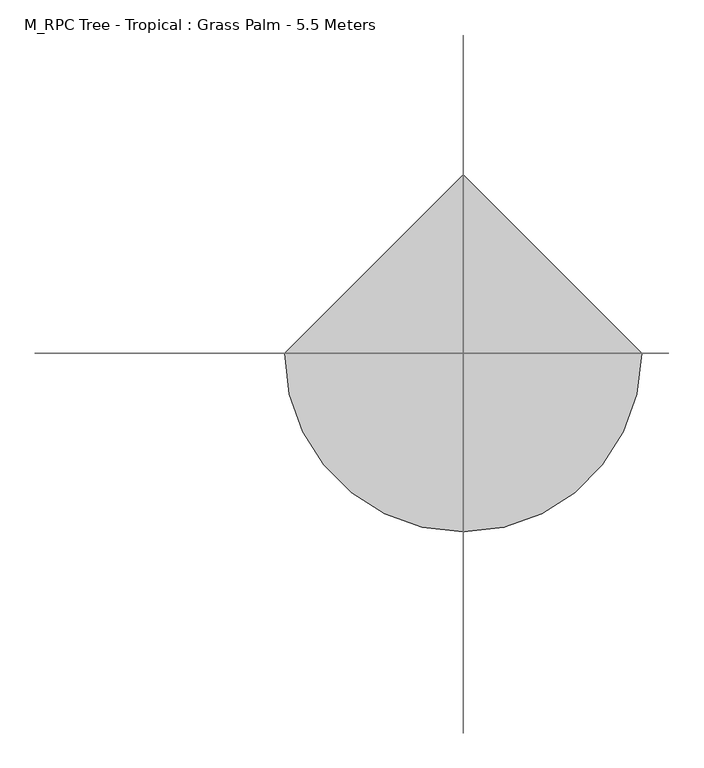
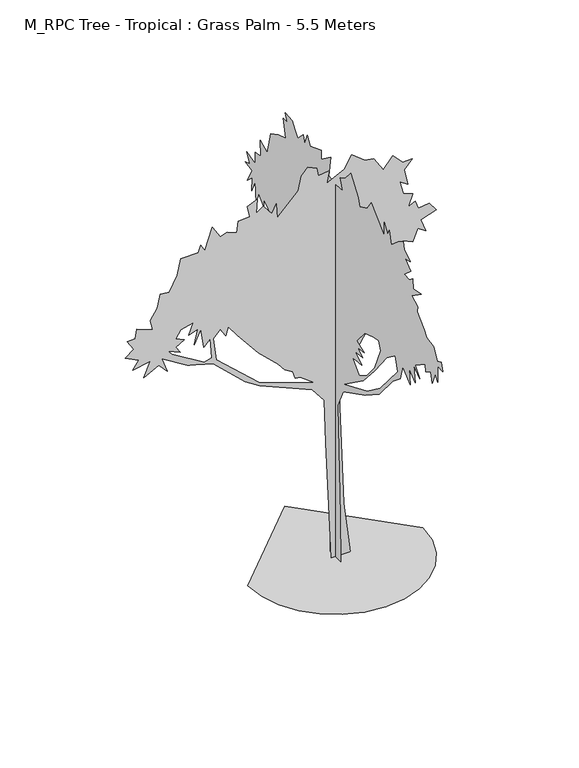
"""IFC4 building model written with IfcOpenShell, lengths in millimetres: geographic element geometry, M_RPC Tree - Tropical : Grass Palm - 5.5 Meters."""

from ifc_helpers import new_model, si_unit, origin, place, context, project, spatial, triangles, source, transform, mapped, element, save


def m_rpc_tree_tropical_grass_palm_5_5_meters_0f61173e(model_context):
    return source(origin(), model_context, "Body", "Tessellation", [
        triangles([(198.5121563, -0.0004669, 0.000137), (109.5820013, -0.0002641, 696.282209), (43.8536913, 0.0002053, 2386.4069527), (410.3796021, 0.0003086, 2969.8983719), (572.0261307, 0.000406, 3417.6646454), (609.3777389, 0.0004587, 3632.4192696), (721.4325634, 0.000452, 3669.7733849), (656.0666405, 0.0004949, 3791.1807999), (749.4469145, 0.0005265, 3959.2618195), (777.4587221, 0.0005019, 3884.5535889), (880.1763622, 0.0005321, 4052.6346085), (1010.9057373, 0.0004946, 3987.2711563), (1076.2717329, 0.0005304, 4155.3521759), (1178.9867569, 0.0004946, 4080.6439453), (1113.6233774, 0.0005527, 4258.0697433), (1319.0559689, 0.0005395, 4323.4331955), (1225.6756222, 0.0005866, 4444.8150307), (1085.6090263, 0.0006027, 4426.1507629), (1042.0062372, 0.0006404, 4540.8870735), (954.8795786, 0.0006402, 4491.5142151), (1010.9057373, 0.0006749, 4650.2504562), (889.3481134, 0.0007069, 4700.3869308), (842.8247177, 0.0007612, 4874.3754387), (945.5397417, 0.0007279, 4808.9864067), (898.8508764, 0.0007933, 5023.7666107), (1001.5685165, 0.0008083, 5135.8289566), (880.1763622, 0.0008266, 5135.8289566), (749.4469145, 0.0008819, 5266.5558609), (628.0548328, 0.0008596, 5117.1393997), (505.3182475, 0.0009317, 5314.2482986), (385.2705606, 0.0009547, 5331.919313), (217.1877242, 0.0010181, 5471.9909958), (114.4714012, 0.000988, 5303.9099762), (-109.6373213, 0.0009913, 5191.8476303), (-81.6239785, 0.0010303, 5350.5838715), (-221.6916826, 0.0010463, 5331.919313), (-240.3675048, 0.0010796, 5443.9816589), (-361.7593503, 0.0011132, 5500.0003326), (-445.7998964, 0.0011005, 5406.6275436), (-483.1515046, 0.0010553, 5219.8569672), (-753.9502007, 0.0010201, 4939.7386002), (-772.6247149, 0.0010762, 5135.8289566), (-828.653417, 0.0010542, 5023.7666107), (-940.7082779, 0.0011092, 5163.8382935), (-1034.0860811, 0.0011055, 5098.4748413), (-1015.4090235, 0.0011535, 5285.2204193), (-1146.140942, 0.001158, 5229.2017456), (-1118.1265909, 0.0011131, 5079.7852844), (-1267.5330963, 0.0011332, 5070.4655045), (-1286.2076832, 0.0010954, 4921.0490433), (-1407.5996922, 0.0011264, 4967.747937), (-1500.9775681, 0.0011329, 4939.7386002), (-1603.6951355, 0.0011941, 5107.8196198), (-1706.4127029, 0.0011309, 4818.3314758), (-1753.1017136, 0.0011633, 4911.7042648), (-1790.4532127, 0.0011436, 4818.3314758), (-2014.5604637, 0.0011774, 4818.3314758), (-2061.249329, 0.0011261, 4603.5768517), (-2163.9668964, 0.0010882, 4407.4609154), (-2285.3590508, 0.0011091, 4416.8059845), (-2322.7106953, 0.0010665, 4239.3798958), (-2416.0885712, 0.0010425, 4099.3337929), (-2382.6964233, 0.0010016, 3967.2572617), (-2593.5117531, 0.0010541, 4043.2895393), (-2612.1760208, 0.0010239, 3921.9077042), (-2714.8935883, 0.0010369, 3912.5629257), (-2630.8658684, 0.0009886, 3781.8360214), (-2742.9029251, 0.0009827, 3697.7827217), (-2565.5024162, 0.0009305, 3604.4099327), (-2640.1853577, 0.0009113, 3492.3475868), (-2416.0885712, 0.0008902, 3539.0464806), (-2500.1287903, 0.0008496, 3342.9564148), (-2304.0361084, 0.0008479, 3445.6739822), (-2191.9813202, 0.000798, 3324.2665672), (-2266.6819931, 0.0008626, 3520.3822128), (-1932.5900311, 0.0007558, 3313.3428154), (-1590.273571, 0.0006787, 3219.8174194), (-1172.1055635, 0.0005081, 2824.7595566), (-982.5363207, 0.0004459, 2701.1877388), (-300.5056764, 0.0002631, 2407.6914093), (-143.5331084, 0.0001855, 2209.3782234), (-126.2243993, 2.09e-05, 1613.6007809), (-53.6101361, -0.0004288, 0.000137), (-1500.9775681, 0.0008979, 3660.4538956), (-1426.2768951, 0.0008562, 3548.3915497), (-1398.2624714, 0.0008824, 3660.4538956), (-1276.8703171, 0.0008209, 3501.6923653), (-1004.3554831, 0.0003611, 3164.2318588), (-746.3927404, 0.0005806, 2912.4030441), (-661.4253977, 0.0005394, 2808.0812141), (-557.8547573, 0.0005067, 2745.340567), (-520.5031128, 0.0004731, 2642.6229996), (-455.1371535, 0.0004607, 2633.2779305), (-268.3816016, 0.0003944, 2493.2088638), (-997.3532215, 0.0005761, 2756.6459816), (-1553.2123158, 0.0007974, 3261.8314247), (-1594.3579147, 0.0008866, 3567.0558174), (-2023.9003006, 0.0008876, 3529.7017021), (-2079.9263866, 0.0009189, 3613.7550018), (-1967.8715984, 0.0009197, 3679.118454), (-2079.9263866, 0.0009519, 3735.136837), (-2014.5604637, 0.00097, 3837.8544044), (-1855.8166649, 0.0009561, 3875.2085197), (-1911.8453671, 0.000924, 3725.8173477), (-1795.9710445, 0.0009167, 3763.5025475), (-1842.3900135, 0.0008704, 3567.2848732), (-1753.1017136, 0.0009076, 3753.8266846), (-1715.750069, 0.0008309, 3492.3475868), (-1631.7095592, 0.0008411, 3576.4008865), (-1612.4492523, 0.0007652, 3307.9445984), (-1712.8319332, 0.0007726, 3279.4007011), (-2135.952618, 0.000907, 3539.0464806), (-2182.6440994, 0.0009293, 3595.0651543), (0.1967722, -126.2945259, 0.0001596), (0.196734, -114.2887362, 634.3486347), (0.1967033, -52.2143547, 2120.548035), (0.1966846, -175.5378682, 2379.5675446), (0.1966095, -673.1974989, 2636.9445671), (0.1965211, -992.9715849, 2843.0418709), (0.1965145, -1302.1785107, 3208.1809204), (0.196489, -1470.9471336, 3342.9564148), (0.1964806, -1526.9732197, 3548.3915497), (0.1964552, -1695.0542393, 3398.9747978), (0.1964594, -1667.0424316, 3604.4099327), (0.1964383, -1807.1091728, 3492.372876), (0.1964439, -1769.7575283, 3716.4725693), (0.1964228, -1909.8242695, 3613.7550018), (0.1964383, -1807.1091728, 3735.136837), (0.1964044, -2031.2188946, 3884.5535889), (0.1964016, -2049.8934814, 3791.1807999), (0.1963861, -2152.6110489, 3847.1994736), (0.1963805, -2189.9600773, 3716.4725693), (0.1963706, -2255.3261456, 3884.5535889), (0.1963607, -2320.6920685, 3809.8450676), (0.1963607, -2320.6920685, 4033.9447609), (0.1963438, -2432.7443859, 4024.6252716), (0.1963495, -2395.3953575, 4136.6623283), (0.1963636, -2302.0150108, 4089.9887238), (0.1963748, -2227.3117218, 4248.7249649), (0.1963988, -2068.5705391, 4276.7340111), (0.1964073, -2012.5418369, 4351.4425323), (0.1963912, -1853.7980381, 4500.8592842), (0.1963898, -1863.1354042, 4575.541935), (0.1964095, -1732.4058838, 4650.2504562), (0.1963771, -1947.175914, 4799.6669174), (0.1964053, -1760.4203075, 4762.3128021), (0.1964067, -1751.0829414, 4893.0397064), (0.196418, -1676.3797977, 4837.0213234), (0.1964349, -1564.3248642, 4846.340522), (0.1964137, -1704.3916054, 4967.747937), (0.1964321, -1583.0019218, 5070.4655045), (0.1964151, -1695.0542393, 5098.4748413), (0.1964363, -1554.9876434, 5182.5028519), (0.1964391, -1536.3105858, 5275.9006393), (0.196456, -1424.2556522, 5210.5371872), (0.19648, -1265.5118534, 5070.4655045), (0.196487, -1218.8229881, 5238.546524), (0.1964927, -1181.4714163, 5163.8382935), (0.1964639, -1106.7706707, 5285.2204193), (0.196504, -1106.7706707, 5098.4748413), (0.1964895, -937.1364029, 5255.9634842), (0.196509, -807.9577326, 5369.2734283), (0.196521, -728.2942812, 5249.9283875), (0.1965471, -555.8361669, 5163.8382935), (0.1965527, -518.4845223, 5266.5558609), (0.1965781, -350.4035028, 5500.0003326), (0.1965964, -229.0103492, 5359.9286499), (0.1966148, -107.618204, 5294.5651978), (0.1966063, -163.6456435, 5145.173735), (0.1966288, -14.2397308, 5135.8289566), (0.1966528, 144.5038522, 5163.8382935), (0.1966472, 107.1527437, 5443.9816589), (0.1966782, 312.5858983, 5294.5651978), (0.1966782, 312.5858983, 5415.9473236), (0.1967163, 564.707464, 5322.5745346), (0.1967261, 630.0734596, 5434.6368805), (0.196736, 695.4368391, 5275.9006393), (0.1967402, 723.4511902, 5378.6182068), (0.1967586, 844.8433445, 5257.2110825), (0.1967684, 910.2093401, 5322.5745346), (0.1967783, 975.5727922, 5425.2921021), (0.1967622, 1134.3165184, 5434.6368805), (0.1967952, 1087.6276531, 5331.919313), (0.1968083, 1174.4359446, 5339.303746), (0.1967995, 1115.6420042, 5098.4748413), (0.1968263, 1293.0603172, 5033.1113892), (0.1968508, 1455.9824947, 4950.7135117), (0.1968629, 1535.8446259, 4640.9053871), (0.1968869, 1694.5882793, 4715.6139084), (0.1968855, 1685.2510586, 4500.8592842), (0.1969038, 1806.6432129, 4482.1694366), (0.1969038, 1806.6432129, 4323.4331955), (0.1969334, 2002.7386562, 4370.1068001), (0.1969223, 1928.9571133, 4250.787339), (0.1969389, 2038.9214767, 4214.579084), (0.1969151, 1881.3465019, 4183.3615128), (0.196932, 1993.4012901, 3987.2711563), (0.1969137, 1872.0091358, 4089.9887238), (0.1969165, 1890.6837227, 3903.2178566), (0.1969038, 1806.6432129, 4080.6439453), (0.196901, 1787.968626, 3800.5002892), (0.1968925, 1731.9399239, 3959.2618195), (0.1968756, 1619.8851357, 3847.1994736), (0.1968756, 1619.8851357, 3949.917041), (0.196869, 1310.8614109, 3745.6530556), (0.1968099, 919.5466335, 3632.4192696), (0.1967908, 792.5526409, 3237.1576401), (0.1967898, 785.995919, 3141.3913925), (0.1967733, 676.7623249, 3072.1575371), (0.1967987, 844.8433445, 2941.4309235), (0.1967817, 732.7884836, 2978.7850388), (0.1968246, 751.4629978, 2782.6946823), (0.1968091, 648.7479738, 2913.4215866), (0.1968063, 630.0734596, 2679.9771149), (0.1968021, 602.0590722, 2782.6946823), (0.1967978, 574.0447211, 2679.9771149), (0.1967908, 527.3558195, 2848.0581345), (0.1967866, 499.3414684, 2689.2966042), (0.1967837, 480.6669542, 2614.6136627), (0.1967781, 443.3153097, 2745.340567), (0.1967682, 377.9493505, 2661.2872673), (0.1967491, 251.276432, 2499.1212936), (0.1966956, 162.3905602, 2114.1747322), (0.1967682, 112.1317639, 1064.5480299), (0.1968089, 116.4897555, 0.0001162), (0.1965757, -631.608831, 2807.9538963), (0.196537, -888.1940414, 3104.5465485), (0.1964954, -1163.6294821, 3449.6205437), (0.1964659, -1358.8922001, 3595.0651543), (0.1964574, -1414.9184315, 3408.3195763), (0.1965169, -1021.2762526, 2939.164492), (0.1965619, -722.832478, 2719.5465019), (0.1966421, -191.6594859, 2493.2088638), (0.1966027, -453.1185631, 2988.104528), (0.1965815, -593.187775, 2997.4493065), (0.1966027, -453.1185631, 3100.1668739), (0.1965773, -621.2021261, 3118.8567215), (0.1965942, -509.0072302, 3191.7316338), (0.1965716, -658.5512272, 3212.2295105), (0.196597, -490.4701713, 3277.5929626), (0.1965705, -666.1620998, 3486.8985008), (0.1965392, -873.3236555, 3557.7363281), (0.1965223, -985.3785164, 3576.4008865), (0.1965161, -1026.231328, 3465.2294746), (0.1965365, -891.2878206, 3143.9121689), (0.1965617, -724.2889297, 2942.0163528), (0.19659, -537.1590729, 2820.0235085), (0.1966111, -397.0924044, 2978.7850388), (-1142.7569189, 0.0, 0.000137), (-1112.5425568, -261.8891381, 0.0001838), (-1026.4879257, -502.3944798, 0.0002268), (-891.4833029, -714.6206245, 0.0002648), (-714.4239796, -891.6799479, 0.0002965), (-502.195255, -1026.6845707, 0.0), (-261.692475, -1112.7392017, 1.54e-05), (0.1967389, -1142.9535639, 2.08e-05), (262.0858013, -1112.7392017, 1.54e-05), (502.5911611, -1026.6845707, 0.0), (714.8172695, -891.6799479, 0.0002965), (891.8765928, -714.6206245, 0.0002648), (1026.8812157, -502.3919363, 0.0002268), (1112.9358467, -261.8891381, 0.0001838), (1143.1502089, 9.99e-05, 0.000137), (0.1965231, 1142.9535639, 0.0002532)], [[95, 110, 96], [86, 3, 87], [87, 3, 88], [88, 3, 89], [106, 105, 107], [89, 3, 90], [90, 3, 91], [74, 73, 75], [42, 41, 43], [14, 13, 15], [98, 113, 99], [72, 71, 73], [96, 110, 97], [110, 109, 97], [70, 69, 71], [24, 23, 25], [26, 25, 27], [85, 84, 86], [55, 54, 56], [53, 52, 54], [104, 103, 105], [10, 9, 11], [108, 107, 109], [100, 99, 101], [46, 45, 47], [47, 45, 48], [66, 65, 67], [68, 67, 69], [16, 15, 17], [17, 15, 18], [35, 34, 36], [73, 71, 75], [64, 63, 65], [7, 6, 8], [3, 86, 4], [19, 18, 20], [32, 31, 33], [1, 83, 2], [83, 82, 2], [2, 82, 3], [82, 81, 3], [28, 27, 29], [12, 11, 13], [81, 80, 3], [4, 86, 5], [5, 86, 6], [21, 20, 22], [44, 43, 45], [27, 25, 29], [25, 23, 29], [60, 59, 61], [99, 113, 101], [49, 48, 50], [57, 56, 58], [6, 86, 8], [38, 37, 39], [37, 36, 39], [39, 36, 40], [36, 34, 40], [65, 63, 67], [67, 63, 69], [69, 63, 71], [71, 63, 75], [92, 91, 93], [91, 3, 93], [93, 3, 94], [3, 80, 94], [80, 79, 94], [94, 79, 95], [79, 78, 95], [95, 78, 110], [78, 77, 110], [110, 77, 111], [77, 76, 111], [111, 76, 112], [76, 75, 112], [112, 75, 113], [75, 63, 113], [113, 63, 101], [101, 63, 102], [97, 109, 84], [109, 107, 84], [8, 86, 9], [63, 62, 102], [62, 61, 102], [61, 59, 102], [102, 59, 103], [59, 58, 103], [58, 56, 103], [56, 54, 103], [18, 15, 20], [15, 13, 20], [13, 11, 20], [54, 52, 103], [52, 51, 103], [51, 50, 103], [103, 50, 105], [105, 50, 107], [107, 50, 84], [84, 50, 86], [86, 50, 9], [50, 48, 9], [48, 45, 9], [40, 34, 41], [30, 29, 31], [31, 29, 33], [33, 29, 34], [11, 9, 20], [29, 23, 34], [23, 22, 34], [34, 22, 41], [22, 20, 41], [20, 9, 41], [9, 45, 41], [45, 43, 41], [226, 245, 246], [245, 226, 227], [233, 116, 117], [126, 127, 128], [209, 210, 211], [198, 199, 200], [213, 214, 215], [196, 197, 198], [226, 246, 247], [200, 201, 202], [144, 145, 146], [238, 239, 240], [194, 195, 196], [218, 219, 220], [215, 216, 217], [158, 159, 160], [211, 212, 213], [245, 227, 228], [244, 245, 228], [131, 132, 133], [236, 237, 238], [234, 235, 236], [122, 123, 124], [133, 134, 135], [124, 125, 126], [156, 157, 158], [233, 226, 247], [192, 193, 194], [202, 203, 204], [151, 152, 153], [171, 172, 173], [175, 176, 177], [233, 117, 118], [232, 233, 118], [232, 118, 119], [231, 232, 119], [231, 119, 120], [230, 231, 120], [230, 120, 121], [217, 218, 220], [230, 121, 122], [229, 230, 122], [146, 147, 148], [177, 178, 179], [181, 182, 183], [188, 189, 190], [135, 136, 137], [135, 137, 138], [213, 215, 217], [173, 174, 175], [153, 154, 155], [183, 184, 185], [129, 130, 131], [165, 166, 167], [149, 150, 151], [161, 162, 163], [180, 181, 183], [192, 194, 196], [225, 114, 115], [224, 225, 115], [224, 115, 116], [223, 224, 116], [156, 158, 160], [233, 247, 248], [180, 183, 185], [179, 180, 185], [209, 211, 213], [167, 168, 169], [165, 167, 169], [164, 165, 169], [190, 191, 192], [248, 234, 236], [222, 223, 116], [222, 116, 233], [196, 198, 200], [222, 233, 248], [221, 222, 248], [220, 221, 248], [142, 143, 144], [217, 220, 248], [192, 196, 200], [151, 153, 155], [151, 155, 156], [149, 151, 156], [243, 244, 228], [243, 228, 229], [144, 146, 148], [144, 148, 149], [217, 248, 236], [138, 139, 140], [207, 208, 209], [200, 202, 204], [192, 200, 204], [190, 192, 204], [188, 190, 204], [188, 204, 205], [188, 205, 206], [209, 213, 217], [209, 217, 236], [209, 236, 238], [209, 238, 240], [207, 209, 240], [206, 207, 240], [206, 240, 241], [188, 206, 241], [187, 188, 241], [186, 187, 241], [185, 186, 241], [179, 185, 241], [177, 179, 241], [175, 177, 241], [173, 175, 241], [171, 173, 241], [170, 171, 241], [169, 170, 241], [164, 169, 241], [164, 241, 242], [164, 242, 243], [163, 164, 243], [161, 163, 243], [160, 161, 243], [160, 243, 229], [156, 160, 229], [149, 156, 229], [144, 149, 229], [142, 144, 229], [141, 142, 229], [141, 229, 122], [141, 122, 124], [141, 124, 126], [141, 126, 128], [141, 128, 129], [140, 141, 129], [138, 140, 129], [138, 129, 131], [138, 131, 133], [138, 133, 135], [263, 264, 249], [262, 263, 249], [262, 249, 250], [261, 262, 250], [261, 250, 251], [261, 251, 252], [260, 261, 252], [259, 260, 252], [259, 252, 253], [259, 253, 254], [259, 254, 255], [259, 255, 256], [259, 256, 257], [259, 257, 258]], closed=False),
    ])


if __name__ == "__main__":
    model = new_model("IFC4")
    model_context = context("Model", 3, world=origin())
    ifc_project = project(units=[si_unit("LENGTHUNIT", "METRE", prefix="MILLI")], contexts=[model_context])
    site = spatial("IfcSite", under=ifc_project)
    building = spatial("IfcBuilding", under=site)
    placement = place(None, origin())
    m_rpc_tree_tropical_grass_palm_5_5_meters_shape = m_rpc_tree_tropical_grass_palm_5_5_meters_0f61173e(model_context)
    element("IfcGeographicElement", 1, ObjectType="M_RPC Tree - Tropical : Grass Palm - 5.5 Meters", at=placement, inside=building, context=model_context, shape_type="MappedRepresentation", body=[
        mapped(m_rpc_tree_tropical_grass_palm_5_5_meters_shape, transform((0.0, 0.0, 0.0), x_axis=(1.0, 0.0, 0.0), y_axis=(0.0, 1.0, 0.0), z_axis=(0.0, 0.0, 1.0))),
    ])
    save(model, "model.ifc")

# Revit data of these elements
# Type "M_RPC Tree - Tropical : Grass Palm - 5.5 Meters"
#   built-in parameter 1005198 = "{2, 15},{39, RPC-16-FXGK-2WG0-PNFG-U000-ST1L-LVER-AU},{1, 0},{1, 0},{2, 35},{1, 8},{5, Color},{1, 0},{1, 0},{3, 0.8},{3, 0.8},{3, 0.8},{1, 8},{7, BBoxMin},{1, 0},{1, 0},{1, 0},{1, 0},{1, 0},{1, 8},{7, BBoxMax},{1, 0},{1, 0},{1, 0},{1, 0},{1, 0},{2, 11},{9, RPCTypeId},{1, 0},{1, 0},{39, RPC-16-FXGK-2WG0-PNFG-U000-ST1L-LVER-AU},{1, 6},{14, RPCPlantHeight},{1, 0},{1, 0},{7, 18.0446},{2, 11},{7, keyword},{1, 0},{1, 0},{76, :Geometry:RPC:Grass Palm:cordyline australis:grass palm:tropical:trees:beach},{2, 11},{8, category},{1, 0},{1, 0},{17, :Trees [Tropical]},{2, 11},{12, LocalizedUID},{1, 0},{1, 0},{10, Grass Palm},{2, 14},{6, Height},{1, 0},{1, 0},{7, 18.0446},{1, 2},{16, Cast Reflections},{1, 0},{1, 0},{1, 0},{1, 2},{12, Cast Shadows},{1, 0},{1, 0},{1, 1},{1, 2},{9, Lock View},{1, 0},{1, 0},{1, 0},{1, 4},{5, ViewC},{1, 0},{1, 0},{1, 0},{2, 11},{20, AdvancedUIDefinition},{1, 0},{1, 0},{0, },{2, 11},{10, AssetLibID},{1, 0},{1, 0},{36, 4D3F6E72-3F99-4203-98E9-AF80B3C7A7A4},{2, 11},{10, BaseSchema},{1, 0},{1, 0},{9, RPCSchema},{2, 11},{12, ExchangeGUID},{1, 0},{1, 0},{0, },{1, 2},{6, Hidden},{1, 0},{1, 0},{1, 0},{1, 4},{11, RPCCategory},{1, 0},{1, 0},{1, 0},{2, 11},{8, RPCImage},{1, 0},{1, 0},{0, },{1, 4},{13, SchemaVersion},{1, 0},{1, 0},{1, 4},{2, 11},{12, UIDefinition},{1, 0},{1, 0},{0, },{2, 11},{6, UIName},{1, 0},{1, 0},{39, RPC-16-FXGK-2WG0-PNFG-U000-ST1L-LVER-AU},{2, 11},{11, VersionGUID},{1, 0},{1, 0},{9, RPCSchema},{2, 11},{9, assettype},{1, 0},{1, 0},{11, RPCGeometry},{2, 11},{11, description},{1, 0},{1, 0},{0, },{2, 11},{9, localname},{1, 0},{1, 0},{3, RPC},{2, 11},{9, localtype},{1, 0},{1, 0},{3, RPC},{1, 4},{8, revision},{1, 0},{1, 0},{1, 1},{2, 11},{9, thumbnail},{1, 0},{1, 0},{0, },{1, 4},{7, version},{1, 0},{1, 0},{1, 1},{1, 2},{20, RPC_Cast Reflections},{1, 0},{1, 0},{1, 1},{1, 2},{16, RPC_Cast Shadows},{1, 0},{1, 0},{1, 1},{1, 2},{13, RPC_Lock View},{1, 0},{1, 0},{1, 0},{1, 4},{9, RPC_ViewC},{1, 0},{1, 0},{1, 0},{21, assetlibrary_base.fbx},{1, 5},"
#   built-in parameter 1005195 = "RPC-16-FXGK-2WG0-PNFG-U000-ST1L-LVER-AU"
#   Type Comments = "Grass Palm"
#   Height = 5500 mm
#   Plan Symbol = element 405753
#   Description = (empty or 0)
#   Default Elevation = 0
